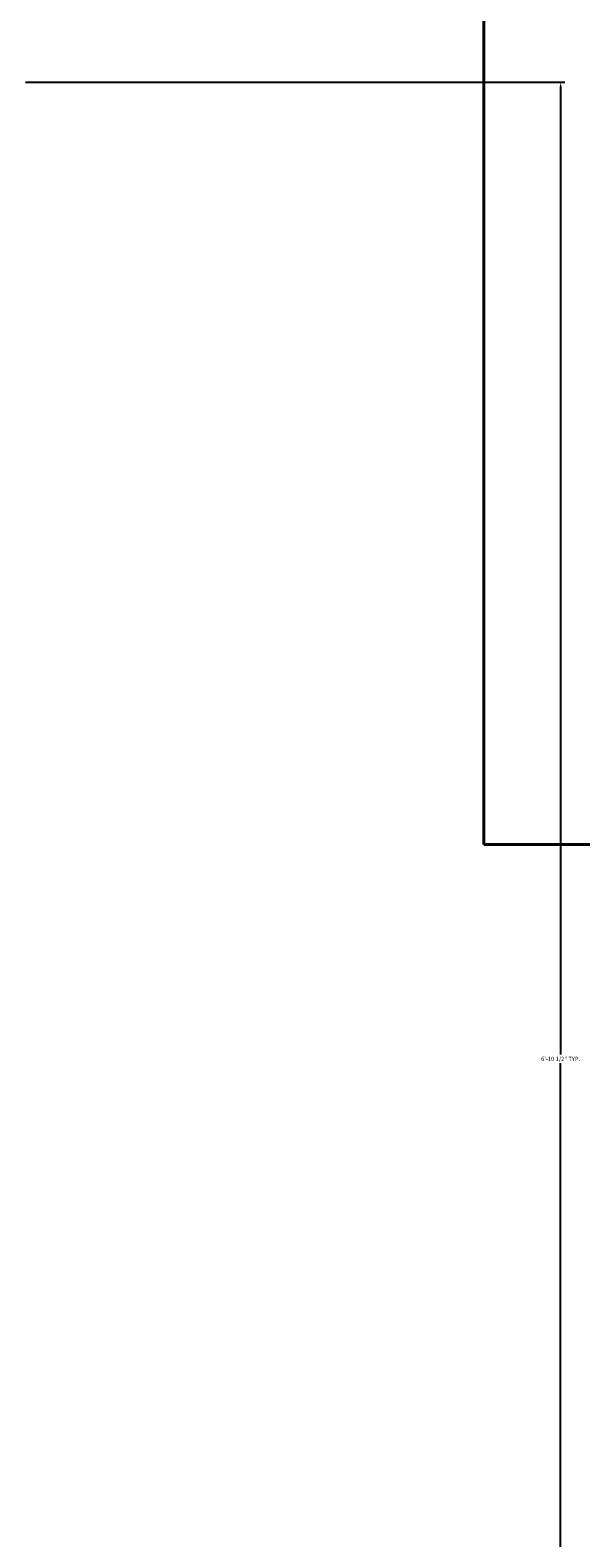
# Model space of a CAD drawing. Units: inches. Extents: x 182 to 1022, y -617 to 111.
# Tile 15 of 33: x 410 to 433, y -276 to -212. Entities that reach past the tile are written whole.
import ezdxf

# ---------------------------------------------------------------- set-up
doc = ezdxf.new("R2010")
doc.units = ezdxf.units.IN
doc.header["$MEASUREMENT"] = 0
doc.layers.add('A-ANNO-DIMS', color=2, linetype='Continuous', lineweight=18)
doc.layers.add('wall', color=1, linetype='Continuous', lineweight=40)
doc.styles.get("Standard").update_dxf_attribs({"font": 'arial.ttf'})
doc.dimstyles.get("Standard").update_dxf_attribs({"dimtxt": 0.18, "dimasz": 0.18, "dimexe": 0.18, "dimexo": 0.0625, "dimgap": 0.09, "dimtad": 0, "dimtih": 1, "dimtoh": 1, "dimdec": 1, "dimzin": 0, "dimdsep": 46, "dimlunit": 4, "dimtxsty": 'Standard', "dimcen": 0.09, "dimadec": 0, "dimazin": 0, "dimtfac": 1, "dimtdec": 1, "dimtofl": 0, "dimtmove": 0, "dimatfit": 3, "dimfxl": 1, "dimtolj": 1, "dimtzin": 0, "dimarcsym": 0})

# ---------------------------------------------------------------- blocks, each defined once
blk = doc.blocks.new('*D27')
at = {"layer": 'A-ANNO-DIMS', "color": 0, "lineweight": -2, "transparency": 16777216}
for p, q in [((409.45, -214.092), (432.299, -214.092)), ((432.119, -214.272), (432.119, -255.274)), ((432.119, -296.642), (432.119, -255.64)), ((409.45, -296.822), (432.299, -296.822))]:
    blk.add_line(p, q, dxfattribs=at)
at = {"layer": 'A-ANNO-DIMS', "color": 0, "transparency": 16777216}
for points in [[(432.089, -214.272), (432.149, -214.272), (432.119, -214.092)], [(432.089, -296.642), (432.149, -296.642), (432.119, -296.822)]]:
    blk.add_solid(points, dxfattribs=at)
at = {"layer": 'Defpoints', "color": 0, "transparency": 16777216}
for p in [(409.388, -214.092), (432.119, -214.092), (409.388, -296.822)]:
    blk.add_point(p, dxfattribs=at)
at = {"layer": 'A-ANNO-DIMS', "color": 0, "transparency": 16777216, "insert": (432.119, -255.457), "char_height": 0.18, "attachment_point": 5}
blk.add_mtext('\\A1;6\'-10 1/2" TYP.', dxfattribs=at)

msp = doc.modelspace()

# ---------------------------------------------------------------- linework, layer by layer
at = {"layer": 'wall'}
for p, q in [((428.861, -121.873), (428.861, -246.373)), ((428.861, -246.373), (433.361, -246.373))]:
    msp.add_line(p, q, dxfattribs=at)

# ---------------------------------------------------------------- dimensions: what is measured, and where the dimension line sits
at = {"layer": 'A-ANNO-DIMS'}
dim = msp.add_linear_dim(base=(432.119, -214.092), p1=(409.388, -296.822), p2=(409.388, -214.092), angle=90, text='<> TYP.', dimstyle='Standard', override={"dimdec": 1, "dimlfac": 1, "dimrnd": 0, "dimzin": 1, "dimdsep": 46, "dimlunit": 4, "dimfrac": 2}, dxfattribs=at)
dim.commit()
dim.dimension.update_dxf_attribs({"geometry": '*D27', "text_midpoint": (432.119, -255.457)})

doc.saveas('drawing.dxf')
